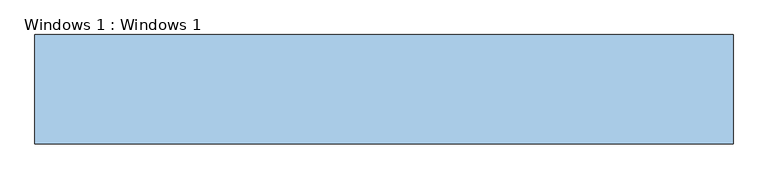
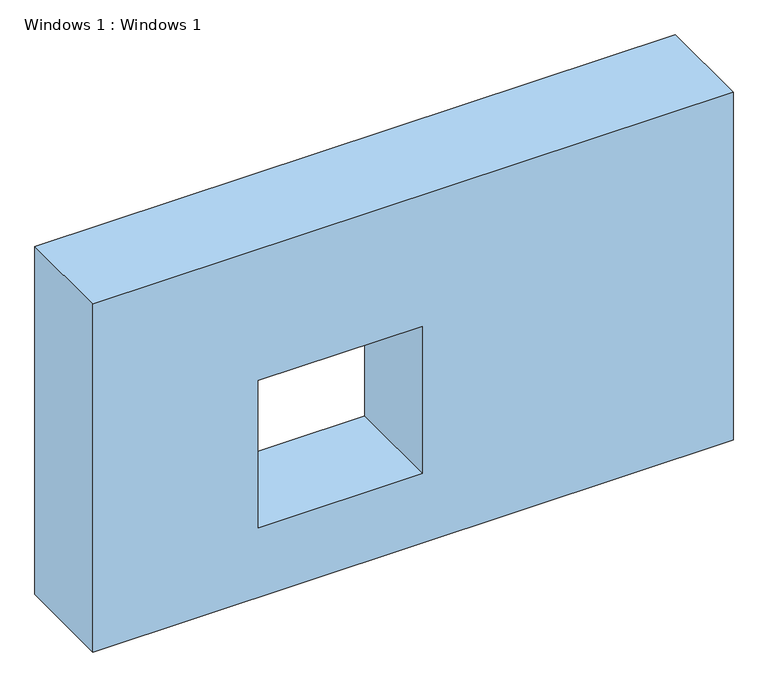
"""IFC4 building model written with IfcOpenShell, lengths in millimetres: window geometry, Windows 1 : Windows 1."""

from ifc_helpers import new_model, si_unit, frame, origin, place, context, project, spatial, polyline, outline, extrude, source, transform, mapped, element, save


def windows_1_windows_1_29d15952(model_context):
    return source(origin(), model_context, "Body", "SweptSolid", [
        extrude(outline(polyline([(3048.0, 3160.1647473), (3048.0, -2143.6852527), (0.0, -2143.6852527), (0.0, 3160.1647473), (3048.0, 3160.1647473)]), holes=[polyline([(1898.65, 586.8147473), (609.6, 586.8147473), (609.6, -772.0852527), (1898.65, -772.0852527), (1898.65, 586.8147473)])]), frame((0.0, 918.057232, 0.0), z_axis=(0.0, 1.0, 0.0), x_axis=(0.0, 0.0, 1.0)), (0.0, 0.0, 1.0), 831.1576125),
    ])


if __name__ == "__main__":
    model = new_model("IFC4")
    model_context = context("Model", 3, world=origin())
    ifc_project = project(units=[si_unit("LENGTHUNIT", "METRE", prefix="MILLI")], contexts=[model_context])
    site = spatial("IfcSite", under=ifc_project)
    building = spatial("IfcBuilding", under=site)
    placement = place(None, origin())
    windows_1_windows_1_shape = windows_1_windows_1_29d15952(model_context)
    element("IfcWindow", 1, ObjectType="Windows 1 : Windows 1", at=placement, inside=building, context=model_context, shape_type="MappedRepresentation", body=[
        mapped(windows_1_windows_1_shape, transform((0.0, 0.0, 0.0), x_axis=(1.0, 0.0, 0.0), y_axis=(0.0, 1.0, 0.0), z_axis=(0.0, 0.0, 1.0))),
    ])
    save(model, "model.ifc")

# Revit data of these elements
# Type "Windows 1 : Windows 1"
#   Type Mark = "25"
